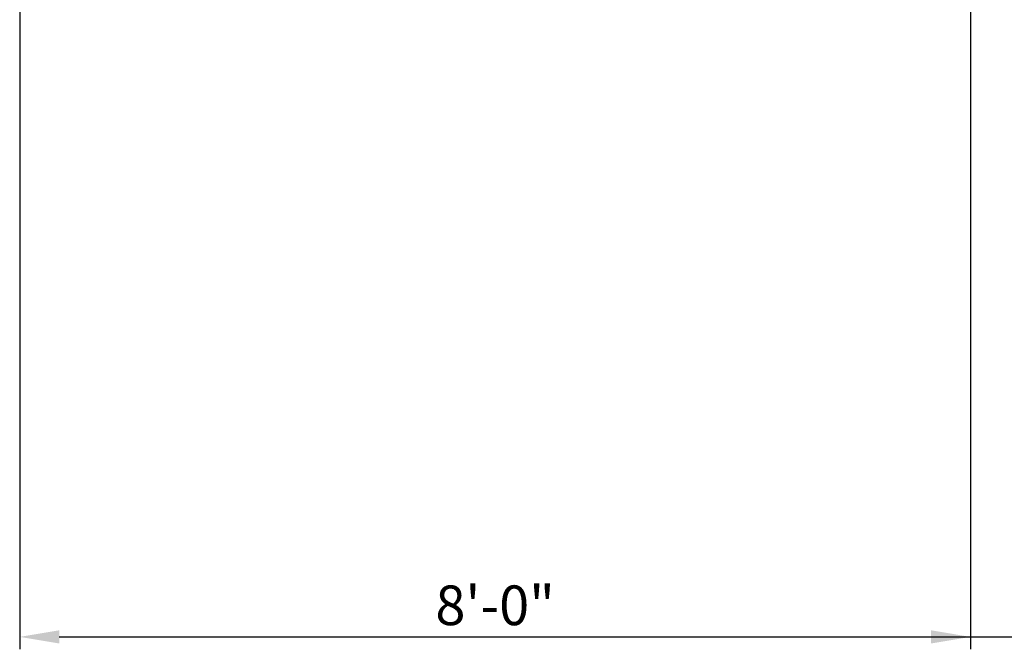
# Model space of a CAD drawing. Units: inches. Extents: x 2091 to 2899, y 967 to 2217.
# Tile 2 of 256: x 2212 to 2312, y 969 to 1033. Entities that reach past the tile are written whole.
import ezdxf

# ---------------------------------------------------------------- set-up
doc = ezdxf.new("R2010")
doc.units = ezdxf.units.IN
doc.layers.add('A-ANNO-DIMS', color=2, linetype='Continuous', lineweight=18)
doc.styles.get("Standard").update_dxf_attribs({"font": 'arial.ttf'})
doc.dimstyles.new('ISO-25', dxfattribs={"dimtxt": 4, "dimasz": 4, "dimexe": 1.25, "dimexo": 0.625, "dimtad": 1, "dimdec": 0, "dimlunit": 3, "dimtxsty": 'Standard', "dimcen": 2.5, "dimadec": 0, "dimazin": 0, "dimtfac": 1, "dimtdec": 0, "dimtmove": 0, "dimatfit": 3, "dimfxl": 1, "dimarcsym": 0})

# ---------------------------------------------------------------- blocks, each defined once
blk = doc.blocks.new('*D71')
at = {"layer": 'A-ANNO-DIMS', "color": 0, "lineweight": -2, "transparency": 16777216}
for p, q in [((2212.144, 1351.294), (2212.144, 969.464)), ((2452.144, 1351.294), (2452.144, 969.464)), ((2216.144, 970.714), (2448.144, 970.714))]:
    blk.add_line(p, q, dxfattribs=at)
at = {"layer": 'A-ANNO-DIMS', "color": 0, "transparency": 16777216}
for points in [[(2216.144, 971.381), (2216.144, 970.048), (2212.144, 970.714)], [(2448.144, 971.381), (2448.144, 970.048), (2452.144, 970.714)]]:
    blk.add_solid(points, dxfattribs=at)
at = {"layer": 'Defpoints', "color": 0, "transparency": 16777216}
for p in [(2212.144, 1351.919), (2452.144, 1351.919), (2452.144, 970.714)]:
    blk.add_point(p, dxfattribs=at)
at = {"layer": 'A-ANNO-DIMS', "color": 0, "transparency": 16777216, "insert": (2332.144, 973.382), "char_height": 4, "attachment_point": 5}
blk.add_mtext('20\'-0"', dxfattribs=at)
blk = doc.blocks.new('*D75')
at = {"layer": 'A-ANNO-DIMS', "color": 0, "lineweight": -2, "transparency": 16777216}
for p, q in [((2212.144, 1274.794), (2212.144, 969.464)), ((2308.144, 1274.794), (2308.144, 969.464)), ((2216.144, 970.714), (2304.144, 970.714))]:
    blk.add_line(p, q, dxfattribs=at)
at = {"layer": 'A-ANNO-DIMS', "color": 0, "transparency": 16777216}
for points in [[(2216.144, 971.381), (2216.144, 970.048), (2212.144, 970.714)], [(2304.144, 971.381), (2304.144, 970.048), (2308.144, 970.714)]]:
    blk.add_solid(points, dxfattribs=at)
at = {"layer": 'Defpoints', "color": 0, "transparency": 16777216}
for p in [(2212.144, 1275.419), (2308.144, 1275.419), (2308.144, 970.714)]:
    blk.add_point(p, dxfattribs=at)
at = {"layer": 'A-ANNO-DIMS', "color": 0, "transparency": 16777216, "insert": (2260.144, 973.382), "char_height": 4, "attachment_point": 5}
blk.add_mtext('8\'-0"', dxfattribs=at)

msp = doc.modelspace()

# ---------------------------------------------------------------- dimensions: what is measured, and where the dimension line sits
at = {"layer": 'A-ANNO-DIMS'}
for base, p1, p2, picture, middle in [((2452.144, 970.714), (2212.144, 1351.919), (2452.144, 1351.919), '*D71', (2332.144, 973.382)), ((2308.144, 970.714), (2212.144, 1275.419), (2308.144, 1275.419), '*D75', (2260.144, 973.382))]:
    dim = msp.add_linear_dim(base=base, p1=p1, p2=p2, dimstyle='ISO-25', override={"dimdec": 1, "dimlfac": 1, "dimrnd": 0, "dimzin": 1, "dimdsep": 46, "dimlunit": 4, "dimfrac": 2}, dxfattribs=at)
    dim.commit()
    dim.dimension.update_dxf_attribs({"geometry": picture, "text_midpoint": middle})

doc.saveas('drawing.dxf')
